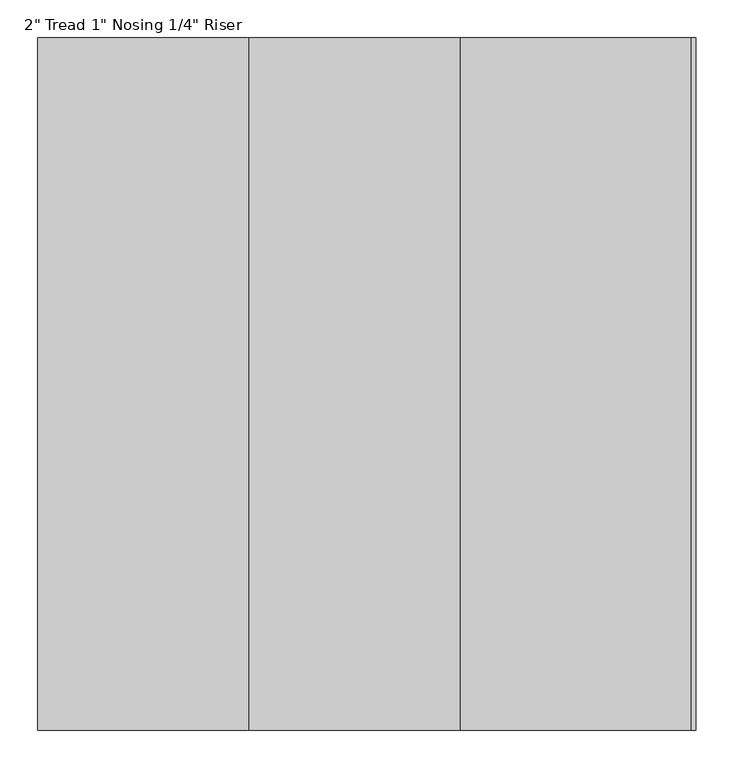
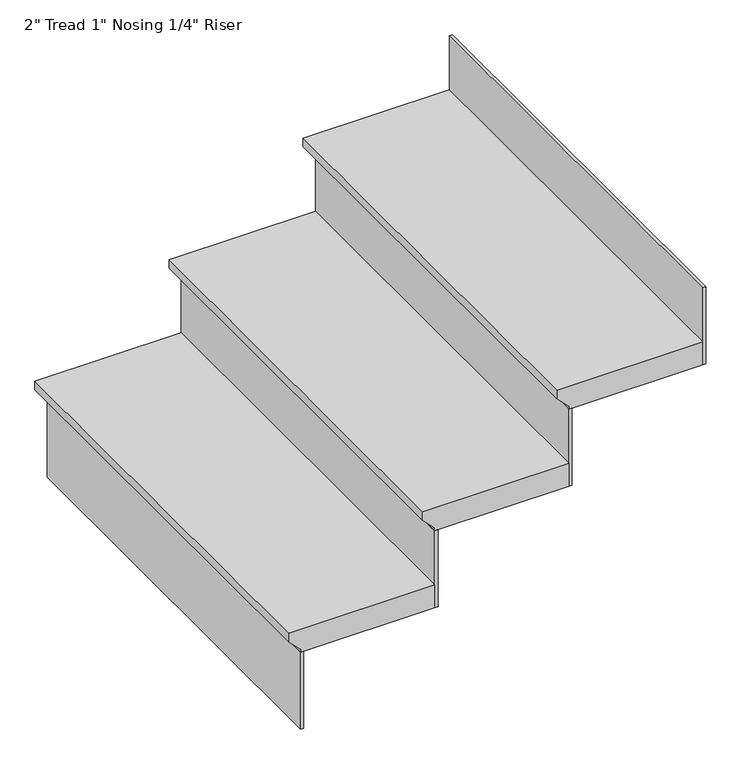
"""IFC4 building model written with IfcOpenShell, lengths in millimetres: stair flight geometry."""

from ifc_helpers import new_model, si_unit, frame, origin, place, context, project, spatial, polyline, outline, extrude, source, transform, mapped, element, save


def stair_flight_812e3324(model_context):
    return source(origin(), model_context, "Body", "SweptSolid", [
        extrude(outline(polyline([(5554.1333333, -9769.5522729), (5554.1333333, -10074.3522729), (5535.0833333, -10074.3522729), (5509.6833333, -10048.9522729), (5503.3333333, -10048.9522729), (5503.3333333, -9769.5522729), (5554.1333333, -9769.5522729)])), frame((0.0, -2916.0844117, 0.0), z_axis=(0.0, 1.0, 0.0), x_axis=(0.0, 0.0, 1.0)), (0.0, 0.0, 1.0), 914.4),
        extrude(outline(polyline([(-10042.6022729, -2916.0844117), (-10048.9522729, -2916.0844117), (-10048.9522729, -2001.6844117), (-10042.6022729, -2001.6844117), (-10042.6022729, -2916.0844117)])), frame((0.0, 0.0, 5334.0), z_axis=(0.0, 0.0, 1.0), x_axis=(1.0, 0.0, 0.0)), (0.0, 0.0, 1.0), 169.3333333),
        extrude(outline(polyline([(-9763.2022729, -2916.0844117), (-9769.5522729, -2916.0844117), (-9769.5522729, -2001.6844117), (-9763.2022729, -2001.6844117), (-9763.2022729, -2916.0844117)])), frame((0.0, 0.0, 5503.3333333), z_axis=(0.0, 0.0, 1.0), x_axis=(1.0, 0.0, 0.0)), (0.0, 0.0, 1.0), 169.3333333),
        extrude(outline(polyline([(5723.4666667, -9490.1522729), (5723.4666667, -9794.9522729), (5704.4166667, -9794.9522729), (5679.0166667, -9769.5522729), (5672.6666667, -9769.5522729), (5672.6666667, -9490.1522729), (5723.4666667, -9490.1522729)])), frame((0.0, -2916.0844117, 0.0), z_axis=(0.0, 1.0, 0.0), x_axis=(0.0, 0.0, 1.0)), (0.0, 0.0, 1.0), 914.4),
        extrude(outline(polyline([(-9483.8022729, -2916.0844117), (-9490.1522729, -2916.0844117), (-9490.1522729, -2001.6844117), (-9483.8022729, -2001.6844117), (-9483.8022729, -2916.0844117)])), frame((0.0, 0.0, 5672.6666667), z_axis=(0.0, 0.0, 1.0), x_axis=(1.0, 0.0, 0.0)), (0.0, 0.0, 1.0), 169.3333333),
        extrude(outline(polyline([(-9204.4022729, -2916.0844117), (-9210.7522729, -2916.0844117), (-9210.7522729, -2001.6844117), (-9204.4022729, -2001.6844117), (-9204.4022729, -2916.0844117)])), frame((0.0, 0.0, 5842.0), z_axis=(0.0, 0.0, 1.0), x_axis=(1.0, 0.0, 0.0)), (0.0, 0.0, 1.0), 169.3333333),
        extrude(outline(polyline([(5892.8, -9210.7522729), (5892.8, -9515.5522729), (5873.75, -9515.5522729), (5848.35, -9490.1522729), (5842.0, -9490.1522729), (5842.0, -9210.7522729), (5892.8, -9210.7522729)])), frame((0.0, -2916.0844117, 0.0), z_axis=(0.0, 1.0, 0.0), x_axis=(0.0, 0.0, 1.0)), (0.0, 0.0, 1.0), 914.4),
    ])


if __name__ == "__main__":
    model = new_model("IFC4")
    model_context = context("Model", 3, world=origin())
    ifc_project = project(units=[si_unit("LENGTHUNIT", "METRE", prefix="MILLI")], contexts=[model_context])
    site = spatial("IfcSite", under=ifc_project)
    building = spatial("IfcBuilding", under=site)
    placement = place(None, origin())
    stair_flight_shape = stair_flight_812e3324(model_context)
    element("IfcStairFlight", 1, ObjectType="2\" Tread 1\" Nosing 1/4\" Riser", at=placement, inside=building, context=model_context, shape_type="MappedRepresentation", body=[
        mapped(stair_flight_shape, transform((0.0, 0.0, 0.0), x_axis=(1.0, 0.0, 0.0), y_axis=(0.0, 1.0, 0.0), z_axis=(0.0, 0.0, 1.0))),
    ])
    save(model, "model.ifc")
